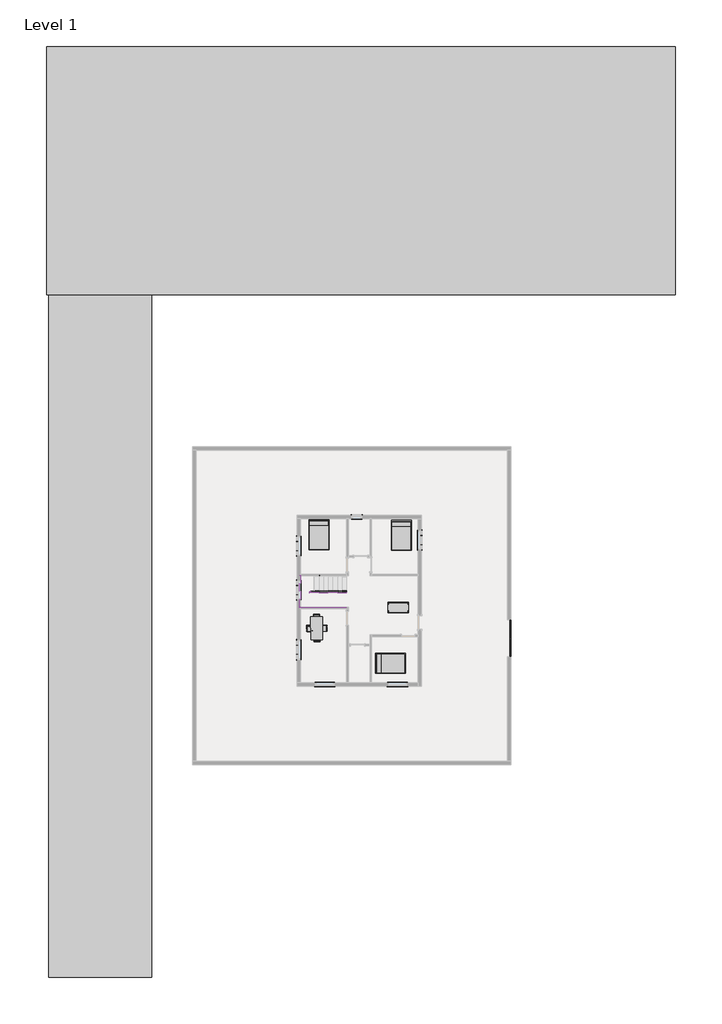
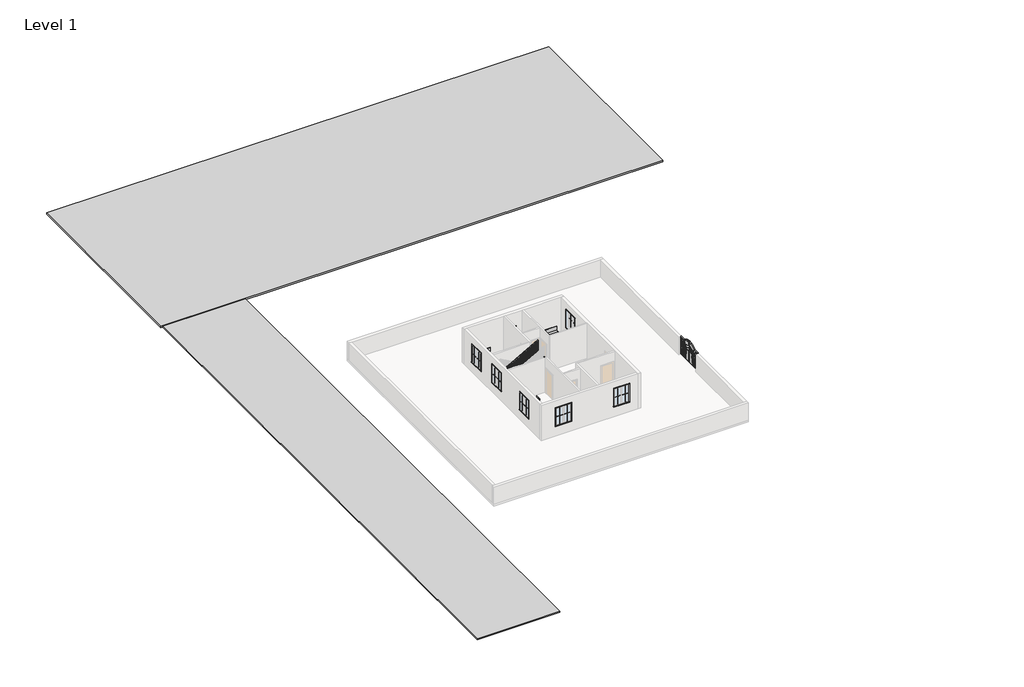
# One storey, part 3 of 3: 31 proxies, 6 members, 4 furniture elements, 1 railing.
"""IFC4 building model written with IfcOpenShell, lengths in millimetres."""

from ifc_helpers import new_model, si_unit, frame, origin, place, context, project, spatial, polyline, outline, extrude, faceted_brep, transform, mapped, element, save
from components import generic_models_1_generic_models_1_08f91587, modern_coffee_table_17989_modern_coffee_table_17989_d3a860c8, muntin_pattern_2x2_muntin_pattern_2x2_6dad3731, muntin_pattern_2x2_muntin_pattern_2x2_a30a3345, muntin_pattern_2x2_muntin_pattern_2x2_53152e2c, muntin_pattern_2x2_muntin_pattern_2x2_e8f3e573, trim_window_exterior_flat_with_sill_92b9b949, trim_window_exterior_flat_with_sill_a665a915, trim_window_interior_flat_picture_frame_3bb882cf, trim_window_interior_flat_picture_frame_d485c387, gate_7956_gate_7956_6bc30956, bed_17739_bed_17739_15c61121, dining_table_w_chairs_11374_0cdfc61b

model = new_model("IFC4")

# Units and contexts
model_context = context("Model", 3, world=origin())
ifc_project = project(units=[si_unit("LENGTHUNIT", "METRE", prefix="MILLI")], contexts=[model_context])

# Site, building, storey
site = spatial("IfcSite", under=ifc_project)
building = spatial("IfcBuilding", under=site)
storey = spatial("IfcBuildingStorey", under=building, Name="Level 1", Elevation=0.0)

# Proxies
placement = place(None, origin())
generic_models_1_generic_models_1_shape = generic_models_1_generic_models_1_08f91587(model_context)
element("IfcBuildingElementProxy", 1, Name="Generic Models 1 : Generic Models 1", ObjectType="Generic Models 1 : Generic Models 1", at=placement, inside=storey, context=model_context, shape_type="MappedRepresentation", body=[
    mapped(generic_models_1_generic_models_1_shape, transform((0.0, 0.0, 0.0), x_axis=(1.0, 0.0, 0.0), y_axis=(0.0, 1.0, 0.0), z_axis=(0.0, 0.0, 1.0))),
])
modern_coffee_table_17989_modern_coffee_table_17989_shape = modern_coffee_table_17989_modern_coffee_table_17989_d3a860c8(model_context)
element("IfcBuildingElementProxy", 2, Name="Modern_Coffee_Table_17989 : Modern_Coffee_Table_17989", ObjectType="Modern_Coffee_Table_17989 : Modern_Coffee_Table_17989", at=placement, inside=storey, context=model_context, shape_type="MappedRepresentation", body=[
    mapped(modern_coffee_table_17989_modern_coffee_table_17989_shape, transform((7937.5, 8234.1992646, 0.0), x_axis=(1.0, 0.0, 0.0), y_axis=(0.0, 1.0, 0.0), z_axis=(0.0, 0.0, 1.0))),
])
muntin_pattern_2x2_muntin_pattern_2x2_shape = muntin_pattern_2x2_muntin_pattern_2x2_6dad3731(model_context)
element("IfcBuildingElementProxy", 3, Name="Muntin Pattern_2x2 : Muntin Pattern_2x2", ObjectType="Muntin Pattern_2x2 : Muntin Pattern_2x2", at=placement, inside=storey, context=model_context, shape_type="MappedRepresentation", body=[
    mapped(muntin_pattern_2x2_muntin_pattern_2x2_shape, transform((7961.3125, 2701.925, 984.25), x_axis=(-1.0, 0.0, 0.0), y_axis=(0.0, -1.0, 0.0), z_axis=(0.0, 0.0, 1.0))),
])
element("IfcBuildingElementProxy", 4, Name="Muntin Pattern_2x2 : Muntin Pattern_2x2", ObjectType="Muntin Pattern_2x2 : Muntin Pattern_2x2", at=placement, inside=storey, context=model_context, shape_type="MappedRepresentation", body=[
    mapped(muntin_pattern_2x2_muntin_pattern_2x2_shape, transform((3154.3625, 2701.925, 984.25), x_axis=(-1.0, 0.0, 0.0), y_axis=(0.0, -1.0, 0.0), z_axis=(0.0, 0.0, 1.0))),
])
element("IfcBuildingElementProxy", 5, Name="Muntin Pattern_2x2 : Muntin Pattern_2x2", ObjectType="Muntin Pattern_2x2 : Muntin Pattern_2x2", at=placement, inside=storey, context=model_context, shape_type="MappedRepresentation", body=[
    mapped(muntin_pattern_2x2_muntin_pattern_2x2_shape, transform((1025.525, 4789.4875, 984.25), x_axis=(0.0, 1.0, 0.0), y_axis=(-1.0, 0.0, 0.0), z_axis=(0.0, 0.0, 1.0))),
])
element("IfcBuildingElementProxy", 6, Name="Muntin Pattern_2x2 : Muntin Pattern_2x2", ObjectType="Muntin Pattern_2x2 : Muntin Pattern_2x2", at=placement, inside=storey, context=model_context, shape_type="MappedRepresentation", body=[
    mapped(muntin_pattern_2x2_muntin_pattern_2x2_shape, transform((1025.525, 8732.8375, 984.25), x_axis=(0.0, 1.0, 0.0), y_axis=(-1.0, 0.0, 0.0), z_axis=(0.0, 0.0, 1.0))),
])
element("IfcBuildingElementProxy", 7, Name="Muntin Pattern_2x2 : Muntin Pattern_2x2", ObjectType="Muntin Pattern_2x2 : Muntin Pattern_2x2", at=placement, inside=storey, context=model_context, shape_type="MappedRepresentation", body=[
    mapped(muntin_pattern_2x2_muntin_pattern_2x2_shape, transform((1025.525, 11637.9625, 984.25), x_axis=(0.0, 1.0, 0.0), y_axis=(-1.0, 0.0, 0.0), z_axis=(0.0, 0.0, 1.0))),
])
element("IfcBuildingElementProxy", 8, Name="Muntin Pattern_2x2 : Muntin Pattern_2x2", ObjectType="Muntin Pattern_2x2 : Muntin Pattern_2x2", at=placement, inside=storey, context=model_context, shape_type="MappedRepresentation", body=[
    mapped(muntin_pattern_2x2_muntin_pattern_2x2_shape, transform((9236.075, 12634.9125, 984.25), x_axis=(0.0, -1.0, 0.0), y_axis=(1.0, 0.0, 0.0), z_axis=(0.0, 0.0, 1.0))),
])
muntin_pattern_2x2_muntin_pattern_2x2_2_shape = muntin_pattern_2x2_muntin_pattern_2x2_a30a3345(model_context)
element("IfcBuildingElementProxy", 9, Name="Muntin Pattern_2x2 : Muntin Pattern_2x2", ObjectType="Muntin Pattern_2x2 : Muntin Pattern_2x2", at=placement, inside=storey, context=model_context, shape_type="MappedRepresentation", body=[
    mapped(muntin_pattern_2x2_muntin_pattern_2x2_2_shape, transform((7354.8875, 2701.925, 984.25), x_axis=(1.0, 0.0, 0.0), y_axis=(0.0, 1.0, 0.0), z_axis=(0.0, 0.0, 1.0))),
])
element("IfcBuildingElementProxy", 10, Name="Muntin Pattern_2x2 : Muntin Pattern_2x2", ObjectType="Muntin Pattern_2x2 : Muntin Pattern_2x2", at=placement, inside=storey, context=model_context, shape_type="MappedRepresentation", body=[
    mapped(muntin_pattern_2x2_muntin_pattern_2x2_2_shape, transform((2547.9375, 2701.925, 984.25), x_axis=(1.0, 0.0, 0.0), y_axis=(0.0, 1.0, 0.0), z_axis=(0.0, 0.0, 1.0))),
])
element("IfcBuildingElementProxy", 11, Name="Muntin Pattern_2x2 : Muntin Pattern_2x2", ObjectType="Muntin Pattern_2x2 : Muntin Pattern_2x2", at=placement, inside=storey, context=model_context, shape_type="MappedRepresentation", body=[
    mapped(muntin_pattern_2x2_muntin_pattern_2x2_2_shape, transform((1025.525, 5395.9125, 984.25), x_axis=(0.0, -1.0, 0.0), y_axis=(1.0, 0.0, 0.0), z_axis=(0.0, 0.0, 1.0))),
])
element("IfcBuildingElementProxy", 12, Name="Muntin Pattern_2x2 : Muntin Pattern_2x2", ObjectType="Muntin Pattern_2x2 : Muntin Pattern_2x2", at=placement, inside=storey, context=model_context, shape_type="MappedRepresentation", body=[
    mapped(muntin_pattern_2x2_muntin_pattern_2x2_2_shape, transform((1025.525, 9339.2625, 984.25), x_axis=(0.0, -1.0, 0.0), y_axis=(1.0, 0.0, 0.0), z_axis=(0.0, 0.0, 1.0))),
])
element("IfcBuildingElementProxy", 13, Name="Muntin Pattern_2x2 : Muntin Pattern_2x2", ObjectType="Muntin Pattern_2x2 : Muntin Pattern_2x2", at=placement, inside=storey, context=model_context, shape_type="MappedRepresentation", body=[
    mapped(muntin_pattern_2x2_muntin_pattern_2x2_2_shape, transform((1025.525, 12244.3875, 984.25), x_axis=(0.0, -1.0, 0.0), y_axis=(1.0, 0.0, 0.0), z_axis=(0.0, 0.0, 1.0))),
])
element("IfcBuildingElementProxy", 14, Name="Muntin Pattern_2x2 : Muntin Pattern_2x2", ObjectType="Muntin Pattern_2x2 : Muntin Pattern_2x2", at=placement, inside=storey, context=model_context, shape_type="MappedRepresentation", body=[
    mapped(muntin_pattern_2x2_muntin_pattern_2x2_2_shape, transform((9236.075, 12028.4875, 984.25), x_axis=(0.0, 1.0, 0.0), y_axis=(-1.0, 0.0, 0.0), z_axis=(0.0, 0.0, 1.0))),
])
muntin_pattern_2x2_muntin_pattern_2x2_3_shape = muntin_pattern_2x2_muntin_pattern_2x2_53152e2c(model_context)
element("IfcBuildingElementProxy", 15, Name="Muntin Pattern_2x2 : Muntin Pattern_2x2", ObjectType="Muntin Pattern_2x2 : Muntin Pattern_2x2", at=placement, inside=storey, context=model_context, shape_type="MappedRepresentation", body=[
    mapped(muntin_pattern_2x2_muntin_pattern_2x2_3_shape, transform((4808.5375, 13960.475, 984.25), x_axis=(1.0, 0.0, 0.0), y_axis=(0.0, 1.0, 0.0), z_axis=(0.0, 0.0, 1.0))),
])
muntin_pattern_2x2_muntin_pattern_2x2_4_shape = muntin_pattern_2x2_muntin_pattern_2x2_e8f3e573(model_context)
element("IfcBuildingElementProxy", 16, Name="Muntin Pattern_2x2 : Muntin Pattern_2x2", ObjectType="Muntin Pattern_2x2 : Muntin Pattern_2x2", at=placement, inside=storey, context=model_context, shape_type="MappedRepresentation", body=[
    mapped(muntin_pattern_2x2_muntin_pattern_2x2_4_shape, transform((5110.1625, 13960.475, 984.25), x_axis=(-1.0, 0.0, 0.0), y_axis=(0.0, -1.0, 0.0), z_axis=(0.0, 0.0, 1.0))),
])
trim_window_exterior_flat_with_sill_shape = trim_window_exterior_flat_with_sill_92b9b949(model_context)
element("IfcBuildingElementProxy", 17, Name="Trim-Window-Exterior-Flat : with Sill", ObjectType="Trim-Window-Exterior-Flat : with Sill", at=placement, inside=storey, context=model_context, shape_type="MappedRepresentation", body=[
    mapped(trim_window_exterior_flat_with_sill_shape, transform((7658.1, 2692.4, 2438.4), x_axis=(1.0, 0.0, 0.0), y_axis=(0.0, 0.0, 1.0), z_axis=(0.0, -1.0, 0.0))),
])
element("IfcBuildingElementProxy", 18, Name="Trim-Window-Exterior-Flat : with Sill", ObjectType="Trim-Window-Exterior-Flat : with Sill", at=placement, inside=storey, context=model_context, shape_type="MappedRepresentation", body=[
    mapped(trim_window_exterior_flat_with_sill_shape, transform((2851.15, 2692.4, 2438.4), x_axis=(1.0, 0.0, 0.0), y_axis=(0.0, 0.0, 1.0), z_axis=(0.0, -1.0, 0.0))),
])
element("IfcBuildingElementProxy", 19, Name="Trim-Window-Exterior-Flat : with Sill", ObjectType="Trim-Window-Exterior-Flat : with Sill", at=placement, inside=storey, context=model_context, shape_type="MappedRepresentation", body=[
    mapped(trim_window_exterior_flat_with_sill_shape, transform((1016.0, 5092.7, 2438.4), x_axis=(0.0, -1.0, 0.0), y_axis=(0.0, 0.0, 1.0), z_axis=(-1.0, 0.0, 0.0))),
])
element("IfcBuildingElementProxy", 20, Name="Trim-Window-Exterior-Flat : with Sill", ObjectType="Trim-Window-Exterior-Flat : with Sill", at=placement, inside=storey, context=model_context, shape_type="MappedRepresentation", body=[
    mapped(trim_window_exterior_flat_with_sill_shape, transform((1016.0, 9036.05, 2438.4), x_axis=(0.0, -1.0, 0.0), y_axis=(0.0, 0.0, 1.0), z_axis=(-1.0, 0.0, 0.0))),
])
element("IfcBuildingElementProxy", 21, Name="Trim-Window-Exterior-Flat : with Sill", ObjectType="Trim-Window-Exterior-Flat : with Sill", at=placement, inside=storey, context=model_context, shape_type="MappedRepresentation", body=[
    mapped(trim_window_exterior_flat_with_sill_shape, transform((1016.0, 11941.175, 2438.4), x_axis=(0.0, -1.0, 0.0), y_axis=(0.0, 0.0, 1.0), z_axis=(-1.0, 0.0, 0.0))),
])
element("IfcBuildingElementProxy", 22, Name="Trim-Window-Exterior-Flat : with Sill", ObjectType="Trim-Window-Exterior-Flat : with Sill", at=placement, inside=storey, context=model_context, shape_type="MappedRepresentation", body=[
    mapped(trim_window_exterior_flat_with_sill_shape, transform((9245.6, 12331.7, 2438.4), x_axis=(0.0, 1.0, 0.0), y_axis=(0.0, 0.0, 1.0), z_axis=(1.0, 0.0, 0.0))),
])
trim_window_exterior_flat_with_sill_2_shape = trim_window_exterior_flat_with_sill_a665a915(model_context)
element("IfcBuildingElementProxy", 23, Name="Trim-Window-Exterior-Flat : with Sill", ObjectType="Trim-Window-Exterior-Flat : with Sill", at=placement, inside=storey, context=model_context, shape_type="MappedRepresentation", body=[
    mapped(trim_window_exterior_flat_with_sill_2_shape, transform((4959.35, 13970.0, 1828.8), x_axis=(-1.0, 0.0, 0.0), y_axis=(0.0, 0.0, 1.0), z_axis=(0.0, 1.0, 0.0))),
])
trim_window_interior_flat_picture_frame_shape = trim_window_interior_flat_picture_frame_3bb882cf(model_context)
element("IfcBuildingElementProxy", 24, Name="Trim-Window-Interior-Flat : Picture Frame", ObjectType="Trim-Window-Interior-Flat : Picture Frame", at=placement, inside=storey, context=model_context, shape_type="MappedRepresentation", body=[
    mapped(trim_window_interior_flat_picture_frame_shape, transform((7658.1, 2921.0, 2438.4), x_axis=(-1.0, 0.0, 0.0), y_axis=(0.0, 0.0, 1.0), z_axis=(0.0, 1.0, 0.0))),
])
element("IfcBuildingElementProxy", 25, Name="Trim-Window-Interior-Flat : Picture Frame", ObjectType="Trim-Window-Interior-Flat : Picture Frame", at=placement, inside=storey, context=model_context, shape_type="MappedRepresentation", body=[
    mapped(trim_window_interior_flat_picture_frame_shape, transform((2851.15, 2921.0, 2438.4), x_axis=(-1.0, 0.0, 0.0), y_axis=(0.0, 0.0, 1.0), z_axis=(0.0, 1.0, 0.0))),
])
element("IfcBuildingElementProxy", 26, Name="Trim-Window-Interior-Flat : Picture Frame", ObjectType="Trim-Window-Interior-Flat : Picture Frame", at=placement, inside=storey, context=model_context, shape_type="MappedRepresentation", body=[
    mapped(trim_window_interior_flat_picture_frame_shape, transform((1244.6, 5092.7, 2438.4), x_axis=(0.0, 1.0, 0.0), y_axis=(0.0, 0.0, 1.0), z_axis=(1.0, 0.0, 0.0))),
])
element("IfcBuildingElementProxy", 27, Name="Trim-Window-Interior-Flat : Picture Frame", ObjectType="Trim-Window-Interior-Flat : Picture Frame", at=placement, inside=storey, context=model_context, shape_type="MappedRepresentation", body=[
    mapped(trim_window_interior_flat_picture_frame_shape, transform((1244.6, 9036.05, 2438.4), x_axis=(0.0, 1.0, 0.0), y_axis=(0.0, 0.0, 1.0), z_axis=(1.0, 0.0, 0.0))),
])
element("IfcBuildingElementProxy", 28, Name="Trim-Window-Interior-Flat : Picture Frame", ObjectType="Trim-Window-Interior-Flat : Picture Frame", at=placement, inside=storey, context=model_context, shape_type="MappedRepresentation", body=[
    mapped(trim_window_interior_flat_picture_frame_shape, transform((1244.6, 11941.175, 2438.4), x_axis=(0.0, 1.0, 0.0), y_axis=(0.0, 0.0, 1.0), z_axis=(1.0, 0.0, 0.0))),
])
element("IfcBuildingElementProxy", 29, Name="Trim-Window-Interior-Flat : Picture Frame", ObjectType="Trim-Window-Interior-Flat : Picture Frame", at=placement, inside=storey, context=model_context, shape_type="MappedRepresentation", body=[
    mapped(trim_window_interior_flat_picture_frame_shape, transform((9017.0, 12331.7, 2438.4), x_axis=(0.0, -1.0, 0.0), y_axis=(0.0, 0.0, 1.0), z_axis=(-1.0, 0.0, 0.0))),
])
trim_window_interior_flat_picture_frame_2_shape = trim_window_interior_flat_picture_frame_d485c387(model_context)
element("IfcBuildingElementProxy", 30, Name="Trim-Window-Interior-Flat : Picture Frame", ObjectType="Trim-Window-Interior-Flat : Picture Frame", at=placement, inside=storey, context=model_context, shape_type="MappedRepresentation", body=[
    mapped(trim_window_interior_flat_picture_frame_2_shape, transform((4959.35, 13741.4, 1828.8), x_axis=(1.0, 0.0, 0.0), y_axis=(0.0, 0.0, 1.0), z_axis=(0.0, -1.0, 0.0))),
])
gate_7956_gate_7956_shape = gate_7956_gate_7956_6bc30956(model_context)
element("IfcBuildingElementProxy", 31, Name="gate_7956 : gate_7956", ObjectType="gate_7956 : gate_7956", at=placement, inside=storey, context=model_context, shape_type="MappedRepresentation", body=[
    mapped(gate_7956_gate_7956_shape, transform((15082.7759659, 5848.35, 0.0), x_axis=(0.0, 1.0, 0.0), y_axis=(-1.0, 0.0, 0.0), z_axis=(0.0, 0.0, 1.0))),
])

# Furniture
bed_17739_bed_17739_shape = bed_17739_bed_17739_15c61121(model_context)
element("IfcFurniture", 32, ObjectType="Bed_17739 : Bed_17739", at=placement, inside=storey, context=model_context, shape_type="MappedRepresentation", body=[
    mapped(bed_17739_bed_17739_shape, transform((2470.15, 12661.9, 0.0), x_axis=(1.0, 0.0, 0.0), y_axis=(0.0, 1.0, 0.0), z_axis=(0.0, 0.0, 1.0))),
])
element("IfcFurniture", 33, ObjectType="Bed_17739 : Bed_17739", at=placement, inside=storey, context=model_context, shape_type="MappedRepresentation", body=[
    mapped(bed_17739_bed_17739_shape, transform((7912.1, 12611.1, 0.0), x_axis=(1.0, 0.0, 0.0), y_axis=(0.0, 1.0, 0.0), z_axis=(0.0, 0.0, 1.0))),
])
element("IfcFurniture", 34, ObjectType="Bed_17739 : Bed_17739", at=placement, inside=storey, context=model_context, shape_type="MappedRepresentation", body=[
    mapped(bed_17739_bed_17739_shape, transform((7207.25, 4197.35, 0.0), x_axis=(0.0, 1.0, 0.0), y_axis=(-1.0, 0.0, 0.0), z_axis=(0.0, 0.0, 1.0))),
])
dining_table_w_chairs_11374_shape = dining_table_w_chairs_11374_0cdfc61b(model_context)
element("IfcFurniture", 35, ObjectType="Dining_Table_w_Chairs_11374", at=placement, inside=storey, context=model_context, shape_type="MappedRepresentation", body=[
    mapped(dining_table_w_chairs_11374_shape, transform((2420.6366388, 6492.5326572, 0.0), x_axis=(-0.019560245774115807, 0.9998086800909743, 0.0), y_axis=(-0.9998086800909743, -0.019560245774115807, 0.0), z_axis=(0.0, 0.0, 1.0))),
])

# Members
element("IfcMember", 36, ObjectType="Stringer - 2\" Width", at=placement, inside=storey, context=model_context, shape_type="SweptSolid", body=[
    extrude(outline(polyline([(0.0, 4295.1355783), (207.5983948, 4295.1355783), (1534.0428392, 1907.5355783), (1185.3641651, 1907.5355783), (0.0, 4041.1910755), (0.0, 4295.1355783)])), frame((0.0, 8893.8068332, 0.0), z_axis=(0.0, 1.0, 0.0), x_axis=(0.0, 0.0, 1.0)), (0.0, 0.0, 1.0), 50.8),
])
element("IfcMember", 37, ObjectType="Stringer - 2\" Width", at=placement, inside=storey, context=model_context, shape_type="SweptSolid", body=[
    extrude(outline(polyline([(1856.7355783, 8944.6068332), (1907.5355783, 8944.6068332), (1907.5355783, 8877.3), (1856.7355783, 8877.3), (1856.7355783, 8944.6068332)])), frame((0.0, 0.0, 1295.4), z_axis=(0.0, 0.0, 1.0), x_axis=(1.0, 0.0, 0.0)), (0.0, 0.0, 1.0), 304.8),
])
element("IfcMember", 38, ObjectType="Stringer - 2\" Width", at=placement, inside=storey, context=model_context, shape_type="SweptSolid", body=[
    extrude(outline(polyline([(1731.5983948, 1856.7355783), (1382.9197207, 1856.7355783), (2737.5863873, 4295.1355783), (3086.2650614, 4295.1355783), (1731.5983948, 1856.7355783)])), frame((0.0, 8826.5, 0.0), z_axis=(0.0, 1.0, 0.0), x_axis=(0.0, 0.0, 1.0)), (0.0, 0.0, 1.0), 50.8),
])
element("IfcMember", 39, ObjectType="Stringer - 2\" Width", at=placement, inside=storey, context=model_context, shape_type="SweptSolid", body=[
    extrude(outline(polyline([(0.0, 4295.1355783), (207.5983948, 4295.1355783), (1600.2, 1788.4526889), (1600.2, 1244.6), (1553.6617086, 1244.6), (0.0, 4041.1910755), (0.0, 4295.1355783)])), frame((0.0, 9969.5, 0.0), z_axis=(0.0, 1.0, 0.0), x_axis=(0.0, 0.0, 1.0)), (0.0, 0.0, 1.0), 50.8),
])
element("IfcMember", 40, ObjectType="Stringer - 2\" Width", at=placement, inside=storey, context=model_context, shape_type="SweptSolid", body=[
    extrude(outline(polyline([(1193.8, 10020.3), (1244.6, 10020.3), (1244.6, 7912.1), (1193.8, 7912.1), (1193.8, 10020.3)])), frame((0.0, 0.0, 1295.4), z_axis=(0.0, 0.0, 1.0), x_axis=(1.0, 0.0, 0.0)), (0.0, 0.0, 1.0), 304.8),
])
element("IfcMember", 41, ObjectType="Stringer - 2\" Width", at=placement, inside=storey, context=model_context, shape_type="SweptSolid", body=[
    extrude(outline(polyline([(1363.3008513, 1193.8), (1295.4, 1193.8), (1295.4, 1699.2000811), (2737.5863873, 4295.1355783), (3086.2650614, 4295.1355783), (1363.3008513, 1193.8)])), frame((0.0, 7861.3, 0.0), z_axis=(0.0, 1.0, 0.0), x_axis=(0.0, 0.0, 1.0)), (0.0, 0.0, 1.0), 50.8),
])

# Railing
element("IfcRailing", 42, ObjectType="Handrail - Rectangular", at=placement, inside=storey, context=model_context, shape_type="SolidModel", body=[
    faceted_brep([(4295.1355783, 8944.6068332, 1083.7333333), (4295.1355783, 8944.6068332, 1025.620221), (4295.1355783, 8995.4068332, 1025.620221), (4295.1355783, 8995.4068332, 1083.7333333), (1932.9355783, 8944.6068332, 2396.0666667), (1882.1355783, 8944.6068332, 2366.1757765), (1882.1355783, 8995.4068332, 2366.1757765), (1932.9355783, 8995.4068332, 2396.0666667), (1932.9355783, 8944.6068332, 2438.4), (1882.1355783, 8944.6068332, 2387.6), (1882.1355783, 8995.4068332, 2387.6), (1932.9355783, 8995.4068332, 2438.4), (1856.7355783, 8944.6068332, 2438.4), (1856.7355783, 8944.6068332, 2387.6), (1805.9355783, 8995.4068332, 2387.6), (1805.9355783, 8995.4068332, 2438.4), (1856.7355783, 8868.4068332, 2438.4), (1856.7355783, 8868.4068332, 2387.6), (1805.9355783, 8868.4068332, 2387.6), (1805.9355783, 8868.4068332, 2438.4), (1856.7355783, 8826.5, 2438.4), (1805.9355783, 8826.5, 2438.4), (1805.9355783, 8775.7, 2387.6), (1856.7355783, 8775.7, 2387.6)], [[[0, 1, 2, 3]], [[1, 0, 4, 5]], [[2, 1, 5, 6]], [[3, 2, 6, 7]], [[0, 3, 7, 4]], [[5, 4, 8, 9]], [[6, 5, 9, 10]], [[7, 6, 10, 11]], [[4, 7, 11, 8]], [[9, 8, 12, 13]], [[10, 9, 13, 14]], [[11, 10, 14, 15]], [[8, 11, 15, 12]], [[13, 12, 16, 17]], [[14, 13, 17, 18]], [[15, 14, 18, 19]], [[12, 15, 19, 16]], [[20, 21, 22, 23]], [[17, 16, 20, 23]], [[18, 17, 23, 22]], [[19, 18, 22, 21]], [[16, 19, 21, 20]]]),
    faceted_brep([(1856.7355783, 8826.5, 2438.4), (1856.7355783, 8775.7, 2387.6), (1805.9355783, 8775.7, 2387.6), (1805.9355783, 8826.5, 2438.4), (1856.7355783, 8826.5, 2549.620221), (1805.9355783, 8826.5, 2579.5111111), (1805.9355783, 8775.7, 2579.5111111), (1856.7355783, 8775.7, 2549.620221)], [[[0, 1, 2, 3]], [[4, 5, 6, 7]], [[1, 0, 4, 7]], [[2, 1, 7, 6]], [[3, 2, 6, 5]], [[0, 3, 5, 4]]]),
    faceted_brep([(1805.9355783, 8826.5, 2579.5111111), (1856.7355783, 8826.5, 2549.620221), (1856.7355783, 8775.7, 2549.620221), (1805.9355783, 8775.7, 2579.5111111), (4295.1355783, 8826.5, 3962.4), (4295.1355783, 8775.7, 3962.4), (4295.1355783, 8775.7, 3904.2868876), (4295.1355783, 8826.5, 3904.2868876)], [[[0, 1, 2, 3]], [[4, 5, 6, 7]], [[1, 0, 4, 7]], [[2, 1, 7, 6]], [[3, 2, 6, 5]], [[0, 3, 5, 4]]]),
    extrude(outline(polyline([(3884.8841099, 4260.2105783), (2878.6666667, 4260.2105783), (2878.6666667, 4279.2605783), (3895.4674432, 4279.2605783), (3884.8841099, 4260.2105783)])), frame((0.0, 8791.575, 0.0), z_axis=(0.0, 1.0, 0.0), x_axis=(0.0, 0.0, 1.0)), (0.0, 0.0, 1.0), 19.05),
    extrude(outline(polyline([(3828.4396654, 4158.6105783), (2878.6666667, 4158.6105783), (2878.6666667, 4177.6605783), (3839.0229988, 4177.6605783), (3828.4396654, 4158.6105783)])), frame((0.0, 8791.575, 0.0), z_axis=(0.0, 1.0, 0.0), x_axis=(0.0, 0.0, 1.0)), (0.0, 0.0, 1.0), 19.05),
    extrude(outline(polyline([(3771.995221, 4057.0105783), (2878.6666667, 4057.0105783), (2878.6666667, 4076.0605783), (3782.5785543, 4076.0605783), (3771.995221, 4057.0105783)])), frame((0.0, 8791.575, 0.0), z_axis=(0.0, 1.0, 0.0), x_axis=(0.0, 0.0, 1.0)), (0.0, 0.0, 1.0), 19.05),
    extrude(outline(polyline([(3715.5507765, 3955.4105783), (2709.3333333, 3955.4105783), (2709.3333333, 3974.4605783), (3726.1341099, 3974.4605783), (3715.5507765, 3955.4105783)])), frame((0.0, 8791.575, 0.0), z_axis=(0.0, 1.0, 0.0), x_axis=(0.0, 0.0, 1.0)), (0.0, 0.0, 1.0), 19.05),
    extrude(outline(polyline([(3659.1063321, 3853.8105783), (2709.3333333, 3853.8105783), (2709.3333333, 3872.8605783), (3669.6896654, 3872.8605783), (3659.1063321, 3853.8105783)])), frame((0.0, 8791.575, 0.0), z_axis=(0.0, 1.0, 0.0), x_axis=(0.0, 0.0, 1.0)), (0.0, 0.0, 1.0), 19.05),
    extrude(outline(polyline([(3602.6618876, 3752.2105783), (2709.3333333, 3752.2105783), (2709.3333333, 3771.2605783), (3613.245221, 3771.2605783), (3602.6618876, 3752.2105783)])), frame((0.0, 8791.575, 0.0), z_axis=(0.0, 1.0, 0.0), x_axis=(0.0, 0.0, 1.0)), (0.0, 0.0, 1.0), 19.05),
    extrude(outline(polyline([(3546.2174432, 3650.6105783), (2540.0, 3650.6105783), (2540.0, 3669.6605783), (3556.8007765, 3669.6605783), (3546.2174432, 3650.6105783)])), frame((0.0, 8791.575, 0.0), z_axis=(0.0, 1.0, 0.0), x_axis=(0.0, 0.0, 1.0)), (0.0, 0.0, 1.0), 19.05),
    extrude(outline(polyline([(3489.7729988, 3549.0105783), (2540.0, 3549.0105783), (2540.0, 3568.0605783), (3500.3563321, 3568.0605783), (3489.7729988, 3549.0105783)])), frame((0.0, 8791.575, 0.0), z_axis=(0.0, 1.0, 0.0), x_axis=(0.0, 0.0, 1.0)), (0.0, 0.0, 1.0), 19.05),
    extrude(outline(polyline([(3433.3285543, 3447.4105783), (2540.0, 3447.4105783), (2540.0, 3466.4605783), (3443.9118876, 3466.4605783), (3433.3285543, 3447.4105783)])), frame((0.0, 8791.575, 0.0), z_axis=(0.0, 1.0, 0.0), x_axis=(0.0, 0.0, 1.0)), (0.0, 0.0, 1.0), 19.05),
    extrude(outline(polyline([(3376.8841099, 3345.8105783), (2370.6666667, 3345.8105783), (2370.6666667, 3364.8605783), (3387.4674432, 3364.8605783), (3376.8841099, 3345.8105783)])), frame((0.0, 8791.575, 0.0), z_axis=(0.0, 1.0, 0.0), x_axis=(0.0, 0.0, 1.0)), (0.0, 0.0, 1.0), 19.05),
    extrude(outline(polyline([(3320.4396654, 3244.2105783), (2370.6666667, 3244.2105783), (2370.6666667, 3263.2605783), (3331.0229988, 3263.2605783), (3320.4396654, 3244.2105783)])), frame((0.0, 8791.575, 0.0), z_axis=(0.0, 1.0, 0.0), x_axis=(0.0, 0.0, 1.0)), (0.0, 0.0, 1.0), 19.05),
    extrude(outline(polyline([(3263.995221, 3142.6105783), (2370.6666667, 3142.6105783), (2370.6666667, 3161.6605783), (3274.5785543, 3161.6605783), (3263.995221, 3142.6105783)])), frame((0.0, 8791.575, 0.0), z_axis=(0.0, 1.0, 0.0), x_axis=(0.0, 0.0, 1.0)), (0.0, 0.0, 1.0), 19.05),
    extrude(outline(polyline([(3207.5507765, 3041.0105783), (2201.3333333, 3041.0105783), (2201.3333333, 3060.0605783), (3218.1341099, 3060.0605783), (3207.5507765, 3041.0105783)])), frame((0.0, 8791.575, 0.0), z_axis=(0.0, 1.0, 0.0), x_axis=(0.0, 0.0, 1.0)), (0.0, 0.0, 1.0), 19.05),
    extrude(outline(polyline([(3151.1063321, 2939.4105783), (2201.3333333, 2939.4105783), (2201.3333333, 2958.4605783), (3161.6896654, 2958.4605783), (3151.1063321, 2939.4105783)])), frame((0.0, 8791.575, 0.0), z_axis=(0.0, 1.0, 0.0), x_axis=(0.0, 0.0, 1.0)), (0.0, 0.0, 1.0), 19.05),
    extrude(outline(polyline([(3094.6618876, 2837.8105783), (2201.3333333, 2837.8105783), (2201.3333333, 2856.8605783), (3105.245221, 2856.8605783), (3094.6618876, 2837.8105783)])), frame((0.0, 8791.575, 0.0), z_axis=(0.0, 1.0, 0.0), x_axis=(0.0, 0.0, 1.0)), (0.0, 0.0, 1.0), 19.05),
    extrude(outline(polyline([(3038.2174432, 2736.2105783), (2032.0, 2736.2105783), (2032.0, 2755.2605783), (3048.8007765, 2755.2605783), (3038.2174432, 2736.2105783)])), frame((0.0, 8791.575, 0.0), z_axis=(0.0, 1.0, 0.0), x_axis=(0.0, 0.0, 1.0)), (0.0, 0.0, 1.0), 19.05),
    extrude(outline(polyline([(2981.7729988, 2634.6105783), (2032.0, 2634.6105783), (2032.0, 2653.6605783), (2992.3563321, 2653.6605783), (2981.7729988, 2634.6105783)])), frame((0.0, 8791.575, 0.0), z_axis=(0.0, 1.0, 0.0), x_axis=(0.0, 0.0, 1.0)), (0.0, 0.0, 1.0), 19.05),
    extrude(outline(polyline([(2925.3285543, 2533.0105783), (2032.0, 2533.0105783), (2032.0, 2552.0605783), (2935.9118876, 2552.0605783), (2925.3285543, 2533.0105783)])), frame((0.0, 8791.575, 0.0), z_axis=(0.0, 1.0, 0.0), x_axis=(0.0, 0.0, 1.0)), (0.0, 0.0, 1.0), 19.05),
    extrude(outline(polyline([(2868.8841099, 2431.4105783), (1862.6666667, 2431.4105783), (1862.6666667, 2450.4605783), (2879.4674432, 2450.4605783), (2868.8841099, 2431.4105783)])), frame((0.0, 8791.575, 0.0), z_axis=(0.0, 1.0, 0.0), x_axis=(0.0, 0.0, 1.0)), (0.0, 0.0, 1.0), 19.05),
    extrude(outline(polyline([(2812.4396654, 2329.8105783), (1862.6666667, 2329.8105783), (1862.6666667, 2348.8605783), (2823.0229988, 2348.8605783), (2812.4396654, 2329.8105783)])), frame((0.0, 8791.575, 0.0), z_axis=(0.0, 1.0, 0.0), x_axis=(0.0, 0.0, 1.0)), (0.0, 0.0, 1.0), 19.05),
    extrude(outline(polyline([(2755.995221, 2228.2105783), (1862.6666667, 2228.2105783), (1862.6666667, 2247.2605783), (2766.5785543, 2247.2605783), (2755.995221, 2228.2105783)])), frame((0.0, 8791.575, 0.0), z_axis=(0.0, 1.0, 0.0), x_axis=(0.0, 0.0, 1.0)), (0.0, 0.0, 1.0), 19.05),
    extrude(outline(polyline([(2699.5507765, 2126.6105783), (1693.3333333, 2126.6105783), (1693.3333333, 2145.6605783), (2710.1341099, 2145.6605783), (2699.5507765, 2126.6105783)])), frame((0.0, 8791.575, 0.0), z_axis=(0.0, 1.0, 0.0), x_axis=(0.0, 0.0, 1.0)), (0.0, 0.0, 1.0), 19.05),
    extrude(outline(polyline([(2643.1063321, 2025.0105783), (1693.3333333, 2025.0105783), (1693.3333333, 2044.0605783), (2653.6896654, 2044.0605783), (2643.1063321, 2025.0105783)])), frame((0.0, 8791.575, 0.0), z_axis=(0.0, 1.0, 0.0), x_axis=(0.0, 0.0, 1.0)), (0.0, 0.0, 1.0), 19.05),
    extrude(outline(polyline([(2586.6618876, 1923.4105783), (1693.3333333, 1923.4105783), (1693.3333333, 1942.4605783), (2597.245221, 1942.4605783), (2586.6618876, 1923.4105783)])), frame((0.0, 8791.575, 0.0), z_axis=(0.0, 1.0, 0.0), x_axis=(0.0, 0.0, 1.0)), (0.0, 0.0, 1.0), 19.05),
    extrude(outline(polyline([(1840.8605783, 8877.9318332), (1840.8605783, 8858.8818332), (1821.8105783, 8858.8818332), (1821.8105783, 8877.9318332), (1840.8605783, 8877.9318332)])), frame((0.0, 0.0, 1524.0), z_axis=(0.0, 0.0, 1.0), x_axis=(1.0, 0.0, 0.0)), (0.0, 0.0, 1.0), 863.6),
    extrude(outline(polyline([(1866.2605783, 8960.4818332), (1847.2105783, 8960.4818332), (1847.2105783, 8979.5318332), (1866.2605783, 8979.5318332), (1866.2605783, 8960.4818332)])), frame((0.0, 0.0, 1524.0), z_axis=(0.0, 0.0, 1.0), x_axis=(1.0, 0.0, 0.0)), (0.0, 0.0, 1.0), 863.6),
    extrude(outline(polyline([(2329.1341099, 1948.8105783), (1354.6666667, 1948.8105783), (1354.6666667, 1967.8605783), (2318.5507765, 1967.8605783), (2329.1341099, 1948.8105783)])), frame((0.0, 8960.4818332, 0.0), z_axis=(0.0, 1.0, 0.0), x_axis=(0.0, 0.0, 1.0)), (0.0, 0.0, 1.0), 19.05),
    extrude(outline(polyline([(2272.6896654, 2050.4105783), (1354.6666667, 2050.4105783), (1354.6666667, 2069.4605783), (2262.1063321, 2069.4605783), (2272.6896654, 2050.4105783)])), frame((0.0, 8960.4818332, 0.0), z_axis=(0.0, 1.0, 0.0), x_axis=(0.0, 0.0, 1.0)), (0.0, 0.0, 1.0), 19.05),
    extrude(outline(polyline([(2216.245221, 2152.0105783), (1354.6666667, 2152.0105783), (1354.6666667, 2171.0605783), (2205.6618876, 2171.0605783), (2216.245221, 2152.0105783)])), frame((0.0, 8960.4818332, 0.0), z_axis=(0.0, 1.0, 0.0), x_axis=(0.0, 0.0, 1.0)), (0.0, 0.0, 1.0), 19.05),
    extrude(outline(polyline([(2159.8007765, 2253.6105783), (1185.3333333, 2253.6105783), (1185.3333333, 2272.6605783), (2149.2174432, 2272.6605783), (2159.8007765, 2253.6105783)])), frame((0.0, 8960.4818332, 0.0), z_axis=(0.0, 1.0, 0.0), x_axis=(0.0, 0.0, 1.0)), (0.0, 0.0, 1.0), 19.05),
    extrude(outline(polyline([(2103.3563321, 2355.2105783), (1185.3333333, 2355.2105783), (1185.3333333, 2374.2605783), (2092.7729988, 2374.2605783), (2103.3563321, 2355.2105783)])), frame((0.0, 8960.4818332, 0.0), z_axis=(0.0, 1.0, 0.0), x_axis=(0.0, 0.0, 1.0)), (0.0, 0.0, 1.0), 19.05),
    extrude(outline(polyline([(2046.9118876, 2456.8105783), (1185.3333333, 2456.8105783), (1185.3333333, 2475.8605783), (2036.3285543, 2475.8605783), (2046.9118876, 2456.8105783)])), frame((0.0, 8960.4818332, 0.0), z_axis=(0.0, 1.0, 0.0), x_axis=(0.0, 0.0, 1.0)), (0.0, 0.0, 1.0), 19.05),
    extrude(outline(polyline([(1990.4674432, 2558.4105783), (1016.0, 2558.4105783), (1016.0, 2577.4605783), (1979.8841099, 2577.4605783), (1990.4674432, 2558.4105783)])), frame((0.0, 8960.4818332, 0.0), z_axis=(0.0, 1.0, 0.0), x_axis=(0.0, 0.0, 1.0)), (0.0, 0.0, 1.0), 19.05),
    extrude(outline(polyline([(1934.0229988, 2660.0105783), (1016.0, 2660.0105783), (1016.0, 2679.0605783), (1923.4396654, 2679.0605783), (1934.0229988, 2660.0105783)])), frame((0.0, 8960.4818332, 0.0), z_axis=(0.0, 1.0, 0.0), x_axis=(0.0, 0.0, 1.0)), (0.0, 0.0, 1.0), 19.05),
    extrude(outline(polyline([(1877.5785543, 2761.6105783), (1016.0, 2761.6105783), (1016.0, 2780.6605783), (1866.995221, 2780.6605783), (1877.5785543, 2761.6105783)])), frame((0.0, 8960.4818332, 0.0), z_axis=(0.0, 1.0, 0.0), x_axis=(0.0, 0.0, 1.0)), (0.0, 0.0, 1.0), 19.05),
    extrude(outline(polyline([(1821.1341099, 2863.2105783), (846.6666667, 2863.2105783), (846.6666667, 2882.2605783), (1810.5507765, 2882.2605783), (1821.1341099, 2863.2105783)])), frame((0.0, 8960.4818332, 0.0), z_axis=(0.0, 1.0, 0.0), x_axis=(0.0, 0.0, 1.0)), (0.0, 0.0, 1.0), 19.05),
    extrude(outline(polyline([(1764.6896654, 2964.8105783), (846.6666667, 2964.8105783), (846.6666667, 2983.8605783), (1754.1063321, 2983.8605783), (1764.6896654, 2964.8105783)])), frame((0.0, 8960.4818332, 0.0), z_axis=(0.0, 1.0, 0.0), x_axis=(0.0, 0.0, 1.0)), (0.0, 0.0, 1.0), 19.05),
    extrude(outline(polyline([(1708.245221, 3066.4105783), (846.6666667, 3066.4105783), (846.6666667, 3085.4605783), (1697.6618876, 3085.4605783), (1708.245221, 3066.4105783)])), frame((0.0, 8960.4818332, 0.0), z_axis=(0.0, 1.0, 0.0), x_axis=(0.0, 0.0, 1.0)), (0.0, 0.0, 1.0), 19.05),
    extrude(outline(polyline([(1651.8007765, 3168.0105783), (677.3333333, 3168.0105783), (677.3333333, 3187.0605783), (1641.2174432, 3187.0605783), (1651.8007765, 3168.0105783)])), frame((0.0, 8960.4818332, 0.0), z_axis=(0.0, 1.0, 0.0), x_axis=(0.0, 0.0, 1.0)), (0.0, 0.0, 1.0), 19.05),
    extrude(outline(polyline([(1595.3563321, 3269.6105783), (677.3333333, 3269.6105783), (677.3333333, 3288.6605783), (1584.7729988, 3288.6605783), (1595.3563321, 3269.6105783)])), frame((0.0, 8960.4818332, 0.0), z_axis=(0.0, 1.0, 0.0), x_axis=(0.0, 0.0, 1.0)), (0.0, 0.0, 1.0), 19.05),
    extrude(outline(polyline([(1538.9118876, 3371.2105783), (677.3333333, 3371.2105783), (677.3333333, 3390.2605783), (1528.3285543, 3390.2605783), (1538.9118876, 3371.2105783)])), frame((0.0, 8960.4818332, 0.0), z_axis=(0.0, 1.0, 0.0), x_axis=(0.0, 0.0, 1.0)), (0.0, 0.0, 1.0), 19.05),
    extrude(outline(polyline([(1482.4674432, 3472.8105783), (508.0, 3472.8105783), (508.0, 3491.8605783), (1471.8841099, 3491.8605783), (1482.4674432, 3472.8105783)])), frame((0.0, 8960.4818332, 0.0), z_axis=(0.0, 1.0, 0.0), x_axis=(0.0, 0.0, 1.0)), (0.0, 0.0, 1.0), 19.05),
    extrude(outline(polyline([(1426.0229988, 3574.4105783), (508.0, 3574.4105783), (508.0, 3593.4605783), (1415.4396654, 3593.4605783), (1426.0229988, 3574.4105783)])), frame((0.0, 8960.4818332, 0.0), z_axis=(0.0, 1.0, 0.0), x_axis=(0.0, 0.0, 1.0)), (0.0, 0.0, 1.0), 19.05),
    extrude(outline(polyline([(1369.5785543, 3676.0105783), (508.0, 3676.0105783), (508.0, 3695.0605783), (1358.995221, 3695.0605783), (1369.5785543, 3676.0105783)])), frame((0.0, 8960.4818332, 0.0), z_axis=(0.0, 1.0, 0.0), x_axis=(0.0, 0.0, 1.0)), (0.0, 0.0, 1.0), 19.05),
    extrude(outline(polyline([(1313.1341099, 3777.6105783), (338.6666667, 3777.6105783), (338.6666667, 3796.6605783), (1302.5507765, 3796.6605783), (1313.1341099, 3777.6105783)])), frame((0.0, 8960.4818332, 0.0), z_axis=(0.0, 1.0, 0.0), x_axis=(0.0, 0.0, 1.0)), (0.0, 0.0, 1.0), 19.05),
    extrude(outline(polyline([(1256.6896654, 3879.2105783), (338.6666667, 3879.2105783), (338.6666667, 3898.2605783), (1246.1063321, 3898.2605783), (1256.6896654, 3879.2105783)])), frame((0.0, 8960.4818332, 0.0), z_axis=(0.0, 1.0, 0.0), x_axis=(0.0, 0.0, 1.0)), (0.0, 0.0, 1.0), 19.05),
    extrude(outline(polyline([(1200.245221, 3980.8105783), (338.6666667, 3980.8105783), (338.6666667, 3999.8605783), (1189.6618876, 3999.8605783), (1200.245221, 3980.8105783)])), frame((0.0, 8960.4818332, 0.0), z_axis=(0.0, 1.0, 0.0), x_axis=(0.0, 0.0, 1.0)), (0.0, 0.0, 1.0), 19.05),
    extrude(outline(polyline([(1143.8007765, 4082.4105783), (169.3333333, 4082.4105783), (169.3333333, 4101.4605783), (1133.2174432, 4101.4605783), (1143.8007765, 4082.4105783)])), frame((0.0, 8960.4818332, 0.0), z_axis=(0.0, 1.0, 0.0), x_axis=(0.0, 0.0, 1.0)), (0.0, 0.0, 1.0), 19.05),
    extrude(outline(polyline([(1087.3563321, 4184.0105783), (169.3333333, 4184.0105783), (169.3333333, 4203.0605783), (1076.7729988, 4203.0605783), (1087.3563321, 4184.0105783)])), frame((0.0, 8960.4818332, 0.0), z_axis=(0.0, 1.0, 0.0), x_axis=(0.0, 0.0, 1.0)), (0.0, 0.0, 1.0), 19.05),
    extrude(outline(polyline([(1840.8605783, 8810.625), (1840.8605783, 8791.575), (1821.8105783, 8791.575), (1821.8105783, 8810.625), (1840.8605783, 8810.625)])), frame((0.0, 0.0, 1524.0), z_axis=(0.0, 0.0, 1.0), x_axis=(1.0, 0.0, 0.0)), (0.0, 0.0, 1.0), 863.6),
    extrude(outline(polyline([(1840.8605783, 8960.4818332), (1821.8105783, 8960.4818332), (1821.8105783, 8979.5318332), (1840.8605783, 8979.5318332), (1840.8605783, 8960.4818332)])), frame((0.0, 0.0, 1524.0), z_axis=(0.0, 0.0, 1.0), x_axis=(1.0, 0.0, 0.0)), (0.0, 0.0, 1.0), 863.6),
    extrude(outline(polyline([(3893.7035543, 4276.0855783), (2878.6666667, 4276.0855783), (2878.6666667, 4295.1355783), (3904.2868876, 4295.1355783), (3893.7035543, 4276.0855783)])), frame((0.0, 8791.575, 0.0), z_axis=(0.0, 1.0, 0.0), x_axis=(0.0, 0.0, 1.0)), (0.0, 0.0, 1.0), 19.05),
    extrude(outline(polyline([(1036.2035543, 4276.0855783), (169.3333333, 4276.0855783), (169.3333333, 4295.1355783), (1025.620221, 4295.1355783), (1036.2035543, 4276.0855783)])), frame((0.0, 8960.4818332, 0.0), z_axis=(0.0, 1.0, 0.0), x_axis=(0.0, 0.0, 1.0)), (0.0, 0.0, 1.0), 19.05),
])

save(model, "model.ifc")

# Revit data of these elements
# Type "Modern_Coffee_Table_17989 : Modern_Coffee_Table_17989"
#   Default Elevation = 0
# Type "Muntin Pattern_2x2 : Muntin Pattern_2x2"
#   Width [instance default] = 4' - 0"
#   Thickness = 0' - 0 1/2"
#   Height [instance default] = 4' - 0"
#   Distance = 0' - 0 3/4"
#   Interior Material [instance default] = none
#   Exterior Material [instance default] = none
#   Default Elevation = 0
# Type "Trim-Window-Exterior-Flat : with Sill"
#   Trim Width = 0' - 2 1/4"
#   Trim Thickness_Picture Frame = 0' - 1 1/4"
#   Trim Thickness_with Sill = 0' - 0 3/4"
#   Sill Thickness = 0' - 1 1/4"
#   Opening Width [instance default] = 2' - 0"
#   Opening Height [instance default] = 3' - 0"
#   Default Elevation = 4' - 0"
#   Sill = yes
#   Picture Frame = no
#   Trim Material [instance default] = none
# Type "Trim-Window-Interior-Flat : Picture Frame"
#   Trim Thickness_Picture Frame = 0' - 1 1/4"
#   Trim Width = 0' - 2 1/4"
#   Trim Thickness_with Sill = 0' - 0 3/4"
#   Sill Thickness = 0' - 1 1/4"
#   Opening Width [instance default] = 2' - 0"
#   Opening Height [instance default] = 3' - 0"
#   Default Elevation = 4' - 0"
#   Sill = no
#   Picture Frame = yes
#   Trim Material [instance default] = none
# Type "gate_7956 : gate_7956"
#   m.s. sheet = none
#   2" x2" pipe = none
#   1"x1"pipe = none
#   Default Elevation = 0
# Type "Bed_17739 : Bed_17739"
#   Default Elevation = 0
# Type "Dining_Table_w_Chairs_11374"
#   Default Elevation = 0
#   Assembly Code = ""
# Type "Handrail - Rectangular"
#   Assembly Code = "C2010400"
#   built-in parameter 1008612 = 0.0416667 (stored number, unit not read)
#   built-in parameter 1008611 = 0.0416667 (stored number, unit not read)
#   built-in parameter 1008609 = 0.333333 (stored number, unit not read)
#   built-in parameter 1008604 = 0.166667 (stored number, unit not read)
#   built-in parameter 1008603 = 0.166667 (stored number, unit not read)
#   Railing Height = 3' - 0"
#   built-in parameter 1008630 = 2
#   built-in parameter 1008610 = 2
#   built-in parameter 1008618 = Baluster - Square : 3/4"
# Element 1 (IfcBuildingElementProxy, "Generic Models 1 : Generic Models 1")
#   Phase Created = New Construction
# Element 2 (IfcBuildingElementProxy, "Modern_Coffee_Table_17989 : Modern_Coffee_Table_17989")
#   Phase Created = New Construction
#   Materials on its faces: "1 Wood", "1 Glass", "1 Metal"
# Elements 3, 4, 5, 6, 7, 8, 9, 10, 11, 12, 13, 14 (IfcBuildingElementProxy, "Muntin Pattern_2x2 : Muntin Pattern_2x2")
#   Width = 1' - 6 5/8"
#   Height = 4' - 6 1/2"
#   Interior Material = Wood - Stained
#   Exterior Material = Clad - White
#   Phase Created = New Construction
#   Materials on its faces: "Clad - White", "Wood - Stained"
# Elements 15, 16 (IfcBuildingElementProxy, "Muntin Pattern_2x2 : Muntin Pattern_2x2")
#   Width = 0' - 6 5/8"
#   Height = 2' - 6 1/2"
#   Interior Material = Wood - Stained
#   Exterior Material = Clad - White
#   Phase Created = New Construction
#   Materials on its faces: "Clad - White", "Wood - Stained"
# Elements 17, 18, 19, 20, 21, 22 (IfcBuildingElementProxy, "Trim-Window-Exterior-Flat : with Sill")
#   Opening Width = 4' - 0"
#   Opening Height = 5' - 0"
#   Trim Material = Clad - White
#   Phase Created = New Construction
#   Materials on its faces: "Clad - White"
# Element 23 (IfcBuildingElementProxy, "Trim-Window-Exterior-Flat : with Sill")
#   Opening Width = 2' - 0"
#   Opening Height = 3' - 0"
#   Trim Material = Clad - White
#   Phase Created = New Construction
#   Materials on its faces: "Clad - White"
# Elements 24, 25, 26, 27, 28, 29 (IfcBuildingElementProxy, "Trim-Window-Interior-Flat : Picture Frame")
#   Opening Width = 4' - 0"
#   Opening Height = 5' - 0"
#   Trim Material = Wood - Stained
#   Phase Created = New Construction
#   Materials on its faces: "Wood - Stained"
# Element 30 (IfcBuildingElementProxy, "Trim-Window-Interior-Flat : Picture Frame")
#   Opening Width = 2' - 0"
#   Opening Height = 3' - 0"
#   Trim Material = Wood - Stained
#   Phase Created = New Construction
#   Materials on its faces: "Wood - Stained"
# Element 31 (IfcBuildingElementProxy, "gate_7956 : gate_7956")
#   Phase Created = New Construction
#   Materials on its faces: "r1"
# Elements 32, 33, 34 (IfcFurniture, "Bed_17739 : Bed_17739")
#   Phase Created = New Construction
#   Materials on its faces: "legs", "sheets", "bed frame", "Blanket"
# Element 35 (IfcFurniture, "Dining_Table_w_Chairs_11374")
#   Phase Created = New Construction
# Elements 36, 37, 38, 39, 40, 41 (IfcMember, "Stringer - 2\" Width")
#   Phase Created = New Construction
# Element 42 (IfcRailing, "Handrail - Rectangular")
#   Phase Created = New Construction
# Materials
#   "1 Wood": class "Glass", colour RGB 81 52 39, transparency 0, Cost = 0
#   "1 Glass": class "Glass", colour RGB 236 240 239, transparency 0.85, Cost = 0
#   "1 Metal": class "Glass", colour RGB 244 244 244, transparency 0, Cost = 0
#   "Clad - White": class "Wood", colour RGB 242 242 238, transparency 0, Cost = 0
#   "Wood - Stained": class "Wood", colour RGB 224 178 126, transparency 0, Cost = 0
#   "r1": class "Generic", colour RGB 120 120 120, transparency 0, Cost = 0
#   "legs": colour RGB 90 73 37, transparency 0, Cost = 0
#   "sheets": colour RGB 200 195 176, transparency 0, Cost = 0
#   "bed frame": colour RGB 90 73 37, transparency 0, Cost = 0
#   "Blanket": class "System", colour RGB 59 0 1, transparency 0, Cost = 0
